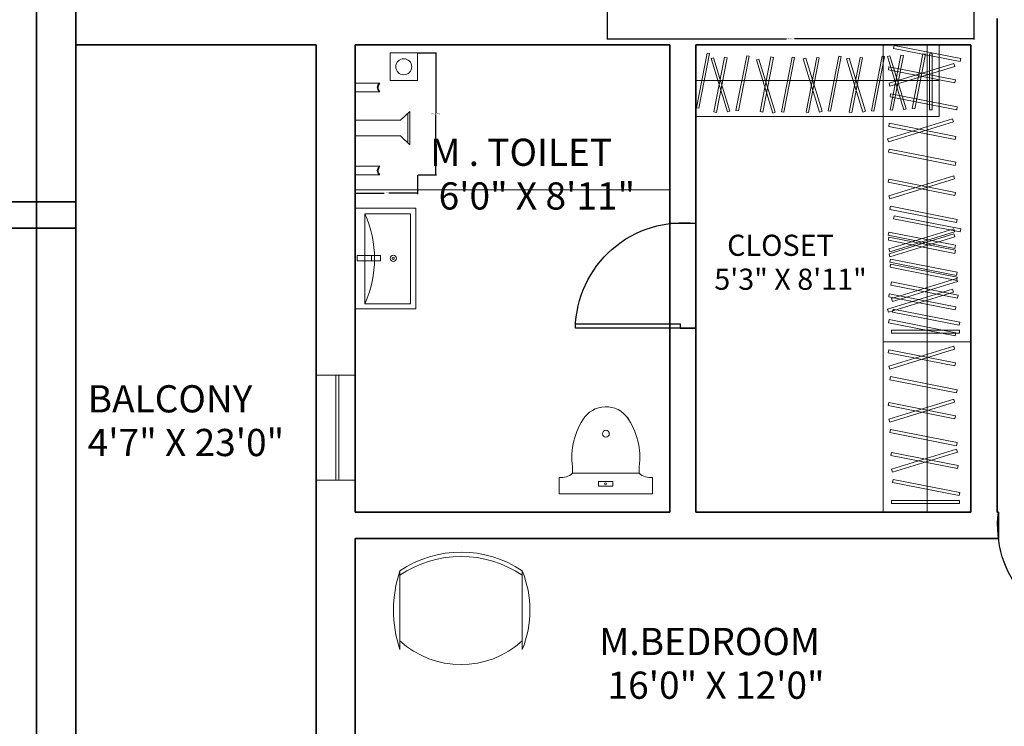
# Model space of a CAD drawing. Units: inches. Extents: x -61 to 1599, y -1316 to 257.
# Tile 160 of 204: x 989 to 1214, y -1101 to -939. Entities that reach past the tile are written whole.
import ezdxf

# ---------------------------------------------------------------- set-up
doc = ezdxf.new("R2010")
doc.units = ezdxf.units.IN
doc.header["$MEASUREMENT"] = 0
doc.linetypes.add('ACAD_ISO02W100', pattern=[15, 12, -3])
for name, color, linetype, lineweight in [('A-ANNO-DIMS', 2, 'Continuous', 18), ('A-AREA-IDEN', 1, 'Continuous', 18), ('A-FLOR-CASE', 8, 'Continuous', 18), ('A-FLOR-FIXT', 8, 'Continuous', 18), ('A-WALL-JAMB', 4, 'ACAD_ISO02W100', 25), ('DOORS', 2, 'Continuous', 25), ('FURNITURE', 83, 'Continuous', 18), ('WALLS', 4, 'Continuous', 35), ('WINDOWS', 220, 'Continuous', 18)]:
    doc.layers.add(name, color=color, linetype=linetype, lineweight=lineweight)
doc.styles.get("Standard").update_dxf_attribs({"font": 'arial.ttf'})
doc.dimstyles.get("Standard").update_dxf_attribs({"dimtxt": 0.18, "dimasz": 0.18, "dimexe": 0.18, "dimexo": 0.0625, "dimgap": 0.09, "dimtad": 0, "dimtih": 1, "dimtoh": 1, "dimdec": 0, "dimzin": 0, "dimdsep": 46, "dimlunit": 3, "dimtxsty": 'Standard', "dimcen": 0.09, "dimadec": 0, "dimazin": 0, "dimtfac": 1, "dimtdec": 0, "dimtofl": 0, "dimtmove": 0, "dimatfit": 3, "dimfxl": 1, "dimtolj": 1, "dimtzin": 0, "dimarcsym": 0})

# ---------------------------------------------------------------- blocks, each defined once
blk = doc.blocks.new('DOOR-SWING-24')
blk.add_line((0, 0), (0, 3.6))
blk.add_lwpolyline([(0, 0), (0, -24), (1.05, -24), (1.05, 0)], close=True)
blk.add_arc((-0.44, 0.62), 24.62, 271.0259, 6.9559)
blk = doc.blocks.new('WIN-24IN')
for p, q in [((0, 4.5), (0, 9)), ((0, 9), (0, 0)), ((24, 9), (24, 0)), ((0, 5.19), (24, 5.19)), ((0, 4.5), (24, 4.5))]:
    blk.add_line(p, q)
blk = doc.blocks.new('WC-FLOOR-MOUNT')
for p, q in [((3.02, 4.69), (3.02, 6.17)), ((3.02, 4.69), (18.31, 4.69)), ((18.31, 4.69), (18.31, 6.17)), ((0, 0), (0, 3.75)), ((21.33, 0), (21.33, 3.75)), ((0, 0), (21.33, 0))]:
    blk.add_line(p, q)
blk.add_lwpolyline([(12.24, 1.73), (8.96, 1.73), (8.96, 2.81), (12.24, 2.81)], close=True)
for centre, radius in [((10.67, 13.73), 0.792), ((10.6, 2.27), 0.208)]:
    blk.add_circle(centre, radius)
for centre, radius, start, end in [((10.67, 13.73), 6.18, 27.6844, 141.4697), ((19.05, 8.26), 16.17, 144.824, 187.4232), ((2.28, 8.26), 16.17, 352.5768, 35.176), ((0.56, 7.25), 3.55, 260.8586, 313.6993), ((20.77, 7.25), 3.55, 226.3007, 279.1414)]:
    blk.add_arc(centre, radius, start, end)
blk = doc.blocks.new('LAVATORY-WALL-2')
blk.add_line((3.67, 10.96), (3.67, 12.19))
for points in [[(0, 23.07), (13.87, 23.07), (13.87, 0), (0, 0)], [(12.66, 21.73), (12.66, 1.19), (2.2, 1.19), (2.2, 21.73)], [(5.78, 12.19), (5.78, 10.96), (0.4, 10.96), (0.4, 12.19)]]:
    blk.add_lwpolyline(points, close=True)
for radius in [0.74, 0.233]:
    blk.add_circle((8.7, 11.57), radius)
blk.add_arc((-20.86, 11.46), 25.25, 335.9939, 24.0061)
blk = doc.blocks.new('SHOWER-FITTINGS-3')
for p, q in [((0, 21.03), (5.62, 21.03)), ((0, 19.05), (5.62, 19.05)), ((10.34, 12.49), (12.46, 14.54)), ((12.05, 14.15), (12.05, 7.29)), ((12.46, 14.54), (12.46, 6.9)), ((0, 12.49), (10.34, 12.49)), ((0, 8.95), (10.34, 8.95)), ((10.34, 8.95), (12.46, 6.9)), ((0, 1.97), (5.62, 1.97)), ((0, 0), (5.62, 0))]:
    blk.add_line(p, q)
blk.add_lwpolyline([(14.24, 21.57), (7.95, 21.57), (7.95, 27.94), (14.24, 27.94)], close=True)
blk.add_circle((11.09, 24.76), 1.83)
for points in [[(5.44, 21.03), (5.24, 20.71), (4.83, 20.05), (5.23, 19.39), (5.44, 19.05)], [(5.62, 21.03), (5.42, 20.71), (5.02, 20.05), (5.42, 19.39), (5.62, 19.05)], [(5.44, 1.97), (5.24, 1.65), (4.83, 1), (5.23, 0.34), (5.44, 0)], [(5.62, 1.97), (5.42, 1.65), (5.02, 1), (5.42, 0.34), (5.62, 0)]]:
    blk.add_open_spline(points, degree=3, knots=[0, 0, 0, 0, 1.043806, 2.132489, 2.132489, 2.132489, 2.132489])
blk = doc.blocks.new('BEDROOM-CHAIR')
for p, q in [((1.45, 3.47), (1.45, 21.47)), ((29.49, 3.47), (29.49, 21.47))]:
    blk.add_line(p, q)
for centre, radius, start, end in [((15.47, 0.83), 24.95, 55.8098, 124.1902), ((15.47, -0.17), 24.95, 55.8098, 124.1902), ((28.58, 12.47), 28.58, 161.6455, 198.3545), ((7.26, 12.47), 23.99, 337.9646, 22.0354), ((15.47, 20.69), 20.68, 227.332, 312.668)]:
    blk.add_arc(centre, radius, start, end)
blk = doc.blocks.new('WARDROBE-HANGING')
blk.add_line((10.05, 0), (10.05, 68))
for points in [[(20.09, 0), (0, 0), (0, 68), (20.09, 68)], [(2.48, 67.85), (17.75, 64.85), (17.61, 64.14), (2.34, 67.15)], [(1.35, 59.16), (16.22, 63.73), (16.43, 63.04), (1.56, 58.47)], [(1.32, 62.96), (16.59, 59.95), (16.45, 59.25), (1.19, 62.25)], [(1.71, 56.78), (16.98, 53.78), (16.84, 53.07), (1.57, 56.08)], [(1, 46.47), (15.87, 51.04), (16.08, 50.35), (1.21, 45.78)], [(1.39, 50.01), (16.66, 47.01), (16.52, 46.3), (1.26, 49.31)], [(1.36, 44.09), (16.63, 41.09), (16.49, 40.38), (1.23, 43.38)], [(1.26, 37.2), (16.53, 34.2), (16.39, 33.49), (1.12, 36.5)], [(1.28, 33.41), (16.16, 37.98), (16.37, 37.29), (1.49, 32.72)], [(1.65, 31.03), (16.92, 28.03), (16.78, 27.32), (1.51, 30.32)], [(1.26, 25.09), (16.53, 22.09), (16.39, 21.38), (1.12, 24.39)], [(1.28, 21.3), (16.15, 25.87), (16.36, 25.18), (1.49, 20.61)], [(1.65, 18.92), (16.91, 15.92), (16.78, 15.21), (1.51, 18.21)], [(1.91, 13.69), (17.17, 10.68), (17.04, 9.98), (1.77, 12.98)], [(1.93, 9.89), (16.8, 14.46), (17.01, 13.77), (2.14, 9.2)], [(2.29, 7.51), (17.56, 4.51), (17.42, 3.8), (2.16, 6.81)], [(17.49, 1.96), (1.93, 1.96), (1.93, 2.68), (17.49, 2.68)]]:
    blk.add_lwpolyline(points, close=True)
blk = doc.blocks.new('WARDROBE-HANGING-2')
blk.add_line((55.7, 8.23), (0, 8.23))
for points in [[(55.7, 16.46), (55.7, 0), (0, 0), (0, 16.46)], [(0.12, 2.03), (2.58, 14.54), (3.16, 14.43), (0.7, 1.92)], [(4.13, 1.08), (6.59, 13.59), (7.17, 13.48), (4.71, 0.97)], [(9.19, 1.4), (11.65, 13.91), (12.23, 13.8), (9.77, 1.29)], [(14.73, 1.14), (17.19, 13.65), (17.77, 13.54), (15.31, 1.03)], [(19.59, 1.12), (22.05, 13.62), (22.63, 13.51), (20.17, 1)], [(25.23, 1.03), (27.69, 13.54), (28.27, 13.43), (25.81, 0.92)], [(30.28, 1.35), (32.74, 13.86), (33.32, 13.75), (30.86, 1.24)], [(35.15, 1.03), (37.61, 13.54), (38.19, 13.42), (35.73, 0.92)], [(40.2, 1.35), (42.66, 13.86), (43.24, 13.74), (40.78, 1.23)], [(47.6, 1.58), (43.86, 13.76), (44.42, 13.94), (48.16, 1.75)], [(44.49, 1.56), (46.95, 14.07), (47.53, 13.95), (45.07, 1.45)], [(49.55, 1.88), (52.01, 14.39), (52.59, 14.27), (50.13, 1.77)], [(54.1, 14.33), (54.1, 1.58), (53.51, 1.58), (53.51, 14.33)], [(7.24, 1.1), (3.5, 13.29), (4.06, 13.46), (7.8, 1.28)], [(17.64, 0.82), (13.9, 13), (14.46, 13.18), (18.2, 0.99)], [(28.34, 1.05), (24.59, 13.24), (25.16, 13.41), (28.9, 1.22)], [(38.26, 1.05), (34.51, 13.23), (35.08, 13.41), (38.82, 1.22)]]:
    blk.add_lwpolyline(points, close=True)
blk = doc.blocks.new('WARDROBE-HANGING-3')
blk.add_line((10.05, 0), (10.05, 68))
blk.add_lwpolyline([(20.09, 68), (20.09, 68), (20.09, 0), (0, 0), (0, 68)])
for points in [[(2.48, 67.85), (17.75, 64.85), (17.61, 64.14), (2.34, 67.15)], [(1.35, 59.16), (16.22, 63.73), (16.43, 63.04), (1.56, 58.47)], [(1.32, 62.96), (16.59, 59.95), (16.45, 59.25), (1.19, 62.25)], [(1.71, 56.78), (16.98, 53.78), (16.84, 53.07), (1.57, 56.08)], [(1, 46.47), (15.87, 51.04), (16.08, 50.35), (1.21, 45.78)], [(1.39, 50.01), (16.66, 47.01), (16.52, 46.3), (1.26, 49.31)], [(1.36, 44.09), (16.63, 41.09), (16.49, 40.38), (1.23, 43.38)], [(1.26, 37.2), (16.53, 34.2), (16.39, 33.49), (1.12, 36.5)], [(1.28, 33.41), (16.16, 37.98), (16.37, 37.29), (1.49, 32.72)], [(1.65, 31.03), (16.92, 28.03), (16.78, 27.32), (1.51, 30.32)], [(1.26, 25.09), (16.53, 22.09), (16.39, 21.38), (1.12, 24.39)], [(1.28, 21.3), (16.15, 25.87), (16.36, 25.18), (1.49, 20.61)], [(1.65, 18.92), (16.91, 15.92), (16.78, 15.21), (1.51, 18.21)], [(1.91, 13.69), (17.17, 10.68), (17.04, 9.98), (1.77, 12.98)], [(1.93, 9.89), (16.8, 14.46), (17.01, 13.77), (2.14, 9.2)], [(2.29, 7.51), (17.56, 4.51), (17.42, 3.8), (2.16, 6.81)], [(17.49, 1.96), (1.93, 1.96), (1.93, 2.68), (17.49, 2.68)]]:
    blk.add_lwpolyline(points, close=True)
blk = doc.blocks.new('*D654')
at = {"layer": 'A-ANNO-DIMS', "color": 0, "lineweight": -2, "transparency": 16777216}
for p, q in [((1080, -947.03), (1084.31, -947.03)), ((1084.13, -947.21), (1084.13, -960.82)), ((1084.13, -974.79), (1084.13, -961.18)), ((1080, -974.97), (1084.31, -974.97))]:
    blk.add_line(p, q, dxfattribs=at)
at = {"layer": 'A-ANNO-DIMS', "color": 0, "transparency": 16777216}
for points in [[(1084.1, -947.21), (1084.16, -947.21), (1084.13, -947.03)], [(1084.1, -974.79), (1084.16, -974.79), (1084.13, -974.97)]]:
    blk.add_solid(points, dxfattribs=at)
at = {"layer": 'DEFPOINTS', "color": 0, "transparency": 16777216}
for p in [(1079.94, -947.03), (1084.13, -947.03), (1079.94, -974.97)]:
    blk.add_point(p, dxfattribs=at)
at = {"layer": 'A-ANNO-DIMS', "color": 0, "transparency": 16777216, "insert": (1084.13, -961), "char_height": 0.18, "attachment_point": 5}
blk.add_mtext('\\A1;SHOWER 28 TYP.', dxfattribs=at)
blk = doc.blocks.new('*D655')
at = {"layer": 'A-ANNO-DIMS', "color": 0, "lineweight": -2, "transparency": 16777216}
for p, q in [((1065.7, -975.03), (1065.7, -979.34)), ((1079.94, -975.03), (1079.94, -979.34)), ((1065.88, -979.16), (1072.3, -979.16)), ((1079.76, -979.16), (1073.34, -979.16))]:
    blk.add_line(p, q, dxfattribs=at)
at = {"layer": 'A-ANNO-DIMS', "color": 0, "transparency": 16777216}
for points in [[(1065.88, -979.13), (1065.88, -979.19), (1065.7, -979.16)], [(1079.76, -979.13), (1079.76, -979.19), (1079.94, -979.16)]]:
    blk.add_solid(points, dxfattribs=at)
at = {"layer": 'DEFPOINTS', "color": 0, "transparency": 16777216}
for p in [(1065.7, -974.97), (1079.94, -974.97), (1079.94, -979.16)]:
    blk.add_point(p, dxfattribs=at)
at = {"layer": 'A-ANNO-DIMS', "color": 0, "transparency": 16777216, "insert": (1072.82, -979.16), "char_height": 0.18, "attachment_point": 5}
blk.add_mtext('\\A1;14 TYP.', dxfattribs=at)
blk = doc.blocks.new('*D684')
at = {"layer": 'A-ANNO-DIMS', "color": 0, "lineweight": -2, "transparency": 16777216}
for p, q in [((1123.37, -931.29), (1123.37, -944.01)), ((1207.37, -931.29), (1207.37, -944.01)), ((1123.55, -943.83), (1164.47, -943.83)), ((1207.19, -943.83), (1166.28, -943.83))]:
    blk.add_line(p, q, dxfattribs=at)
at = {"layer": 'A-ANNO-DIMS', "color": 0, "transparency": 16777216}
for points in [[(1123.55, -943.8), (1123.55, -943.86), (1123.37, -943.83)], [(1207.19, -943.8), (1207.19, -943.86), (1207.37, -943.83)]]:
    blk.add_solid(points, dxfattribs=at)
at = {"layer": 'DEFPOINTS', "color": 0, "transparency": 16777216}
for p in [(1123.37, -931.23), (1207.37, -931.23), (1207.37, -943.83)]:
    blk.add_point(p, dxfattribs=at)
at = {"layer": 'A-ANNO-DIMS', "color": 0, "transparency": 16777216, "insert": (1165.37, -943.83), "char_height": 0.18, "attachment_point": 5}
blk.add_mtext('\\A1;SOFA 84 TYP.', dxfattribs=at)

msp = doc.modelspace()

# ---------------------------------------------------------------- linework, layer by layer
at = {"layer": 'A-FLOR-FIXT'}
msp.add_line((1065.7028, -978.3552), (1137.7028, -978.3552), dxfattribs=at)
at = {"layer": 'A-WALL-JAMB'}
for p, q in [((1143.7028, -986.083), (1137.7028, -986.083)), ((1143.7028, -1010.083), (1137.7028, -1010.083)), ((1212.999, -1052.169), (1212.999, -1058.169))]:
    msp.add_line(p, q, dxfattribs=at)
at = {"layer": 'WALLS'}
for p, q in [((992.7028, -1211.169), (992.7028, -741.169)), ((1001.7028, -1202.169), (1001.7028, -777.169)), ((1212.7028, -1052.169), (1212.7028, -939.169)), ((1001.7028, -945.169), (1056.7028, -945.169)), ((1056.7028, -945.169), (1056.7028, -1202.169)), ((1065.7028, -945.169), (1137.7028, -945.169)), ((1065.7028, -1052.169), (1065.7028, -945.169)), ((1137.7028, -1052.169), (1137.7028, -945.169)), ((1143.7028, -945.169), (1206.7028, -945.169)), ((1143.7028, -1052.169), (1143.7028, -945.169)), ((1206.7028, -1052.169), (1206.7028, -945.169)), ((1001.7028, -981.169), (835.7028, -981.169)), ((1001.7028, -987.169), (835.7028, -987.169)), ((1065.7028, -1052.169), (1137.7028, -1052.169)), ((1143.7028, -1052.169), (1206.7028, -1052.169)), ((1212.7028, -1052.169), (1212.999, -1052.169)), ((1065.7028, -1058.169), (1065.7028, -1202.169)), ((1065.7028, -1058.169), (1213.0034, -1058.169))]:
    msp.add_line(p, q, dxfattribs=at)

# ---------------------------------------------------------------- block references
at = {"layer": 'A-FLOR-CASE'}
for name, p in [('WARDROBE-HANGING-2', (1143.703, -961.6291)), ('WARDROBE-HANGING', (1186.609, -1013.1691)), ('WARDROBE-HANGING-3', (1186.609, -1052.1691))]:
    msp.add_blockref(name, p, dxfattribs=at)
at = {"layer": 'A-FLOR-FIXT'}
for name, p in [('SHOWER-FITTINGS-3', (1065.703, -974.9701)), ('LAVATORY-WALL-2', (1065.703, -1005.6301)), ('WC-FLOOR-MOUNT', (1112.4199, -1047.9386))]:
    msp.add_blockref(name, p, dxfattribs=at)
at = {"layer": 'DOORS', "extrusion": (0, 0, -1), "zscale": -1, "rotation": 90.0000000000004}
msp.add_blockref('DOOR-SWING-24', (-1140.1028, -1010.083), dxfattribs=at)
at = {"layer": 'DOORS', "extrusion": (0, 0, -1), "zscale": -1}
msp.add_blockref('DOOR-SWING-24', (-1236.999, -1055.769), dxfattribs=at)
at = {"layer": 'FURNITURE'}
msp.add_blockref('BEDROOM-CHAIR', (1074.4434, -1087.064), dxfattribs=at)
at = {"layer": 'WINDOWS', "rotation": 269.9999999999999}
msp.add_blockref('WIN-24IN', (1056.7027, -1020.8394), dxfattribs=at)

# ---------------------------------------------------------------- texts
at = {"layer": 'A-AREA-IDEN'}
for s, height, p in [(' M . TOILET', 6.223643, (1080.978, -972.8968)), ('  6\'0" X 8\'11"', 6.223643, (1080.978, -982.8945)), ('  CLOSET', 4.8321, (1147.9149, -993.4918)), ('5\'3" X 8\'11"', 4.832098, (1147.9149, -1001.2541)), ('BALCONY', 6.22364, (1004.4051, -1029.3256)), ('4\'7" X 23\'0"', 6.223643, (1004.4051, -1039.3233)), ('M.BEDROOM ', 6.22364, (1121.5758, -1084.8688)), (' 16\'0" X 12\'0"', 6.223643, (1121.5758, -1094.8665))]:
    msp.add_text(s, height=height, dxfattribs=at).set_placement(p)

# ---------------------------------------------------------------- dimensions: what is measured, and where the dimension line sits
at = {"layer": 'A-ANNO-DIMS'}
for base, p1, p2, text, picture, middle in [((1207.3746, -943.8253), (1123.3746, -931.2253), (1207.3746, -931.2253), 'SOFA <> TYP.', '*D684', (1165.3746, -943.8253)), ((1079.9412, -979.1612), (1065.7028, -974.9705), (1079.9412, -974.9705), '<> TYP.', '*D655', (1072.822, -979.1612))]:
    dim = msp.add_linear_dim(base=base, p1=p1, p2=p2, text=text, dimstyle='Standard', override={"dimdec": 0, "dimlfac": 1, "dimrnd": 0, "dimzin": 0, "dimdsep": 46, "dimlunit": 2}, dxfattribs=at)
    dim.commit()
    dim.dimension.update_dxf_attribs({"geometry": picture, "text_midpoint": middle})
dim = msp.add_linear_dim(base=(1084.1319, -947.0326), p1=(1079.9412, -974.9705), p2=(1079.9412, -947.0326), angle=90, text='SHOWER <> TYP.', dimstyle='Standard', override={"dimdec": 0, "dimlfac": 1, "dimrnd": 0, "dimzin": 0, "dimdsep": 46, "dimlunit": 2}, dxfattribs=at)
dim.commit()
dim.dimension.update_dxf_attribs({"geometry": '*D654', "text_midpoint": (1084.1319, -961.0016)})

doc.saveas('drawing.dxf')
